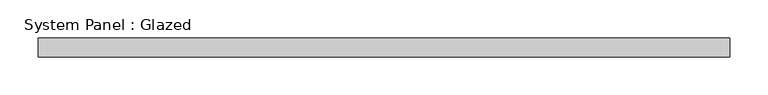
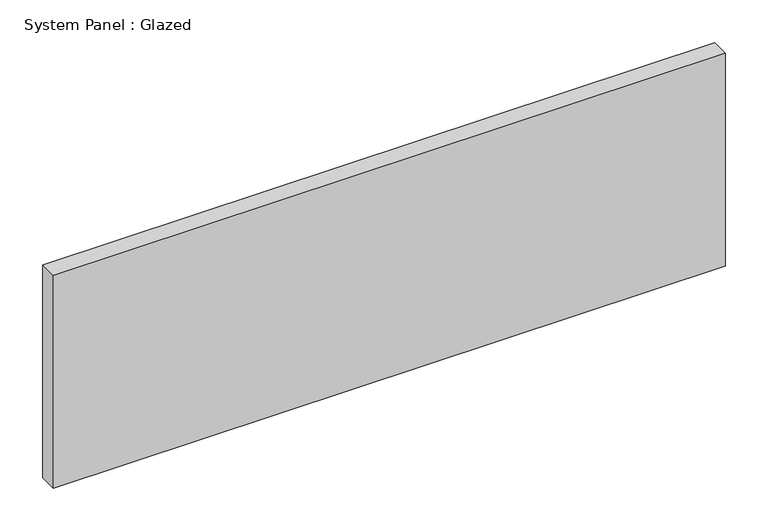
"""IFC4 building model written with IfcOpenShell, lengths in millimetres: plate geometry, System Panel : Glazed."""

from ifc_helpers import new_model, si_unit, origin, origin_with_axes, place, context, project, spatial, polyline, outline, extrude, source, transform, mapped, element, save


def system_panel_glazed_2e822fb3(model_context):
    return source(origin(), model_context, "Body", "SweptSolid", [
        extrude(outline(polyline([(455.0137276, 24.5), (-455.0137276, 24.5), (-455.0137276, 49.5), (455.0137276, 49.5), (455.0137276, 24.5)])), origin_with_axes(), (0.0, 0.0, 1.0), 304.8),
    ])


if __name__ == "__main__":
    model = new_model("IFC4")
    model_context = context("Model", 3, world=origin())
    ifc_project = project(units=[si_unit("LENGTHUNIT", "METRE", prefix="MILLI")], contexts=[model_context])
    site = spatial("IfcSite", under=ifc_project)
    building = spatial("IfcBuilding", under=site)
    placement = place(None, origin())
    system_panel_glazed_shape = system_panel_glazed_2e822fb3(model_context)
    element("IfcPlate", 1, ObjectType="System Panel : Glazed", at=placement, inside=building, context=model_context, shape_type="MappedRepresentation", body=[
        mapped(system_panel_glazed_shape, transform((0.0, 0.0, 0.0), x_axis=(1.0, 0.0, 0.0), y_axis=(0.0, 1.0, 0.0), z_axis=(0.0, 0.0, 1.0))),
    ])
    save(model, "model.ifc")

# Revit data of these elements
# Type "System Panel : Glazed"
#   Keynote = "H11"
#   Construction Type Id = "GSP4R"
#   Analytic Construction = "1/8 in Pilkington single glazing"
#   Visual Light Transmittance = 0.9
#   Solar Heat Gain Coefficient = 0.86
#   Heat Transfer Coefficient (U) = 6.7069 W/(m²·K)
#   Define Thermal Properties by = 1
# Element 1 (IfcPlate, "System Panel : Glazed")
#   Materials on its faces: "Glass"
# Materials
#   "Glass": class "Glass", colour RGB 0 128 192, transparency 0.9, Description = "Soda Lime Glass", Cost = 0
